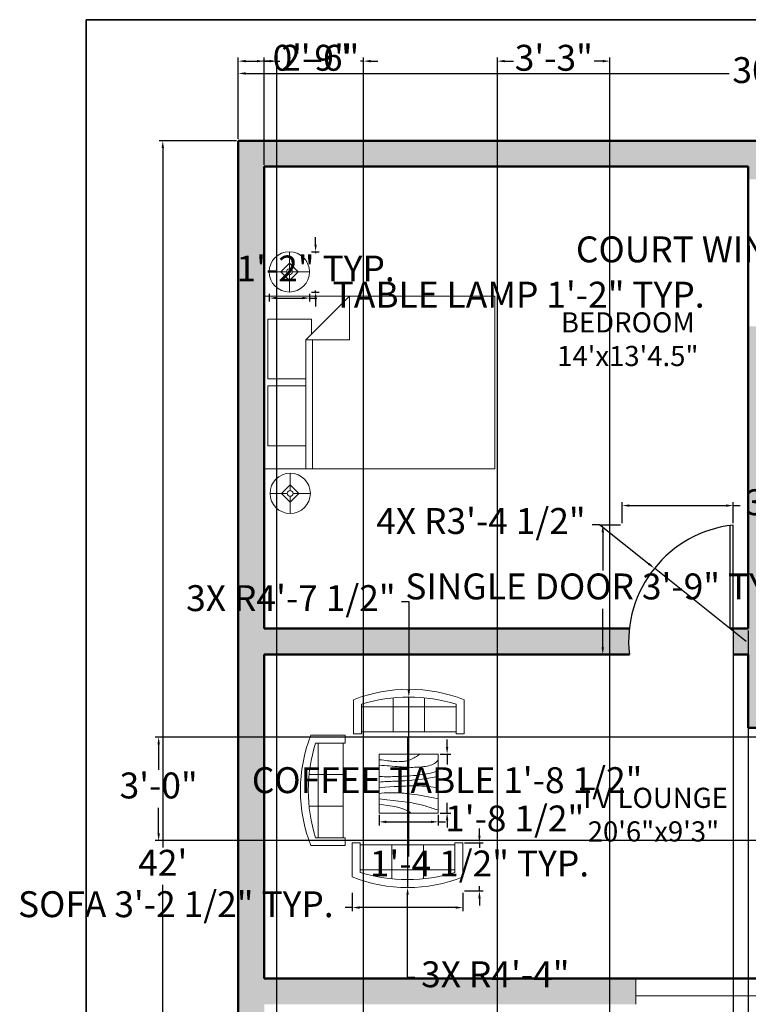
# Model space of a CAD drawing. Units: inches. Extents: x 3695 to 4182, y 4462 to 5050.
# Tile 2 of 3: x 3695 to 3948, y 4708 to 5050. Entities that reach past the tile are written whole.
import ezdxf

# ---------------------------------------------------------------- set-up
doc = ezdxf.new("R2010")
doc.units = ezdxf.units.IN
for name, color, linetype, lineweight in [('A-ANNO-DIMS', 2, 'Continuous', 18), ('A-ANNO-TTLB', 7, 'Continuous', 35), ('A-AREA-IDEN', 7, 'Continuous', 25), ('A-DOOR', 3, 'Continuous', 25), ('A-FURN', 8, 'Continuous', 18), ('A-GLAZ', 4, 'Continuous', 18), ('A-WALL', 7, 'Continuous', 50)]:
    doc.layers.add(name, color=color, linetype=linetype, lineweight=lineweight)
doc.layers.add('A-WALL-PATT', color=18, linetype='Continuous', lineweight=13, true_color=0x000000)
doc.styles.get("Standard").update_dxf_attribs({"font": 'arial.ttf'})
doc.dimstyles.new('ISO-25', dxfattribs={"dimtxt": 9, "dimasz": 2.5, "dimexe": 1.25, "dimexo": 0.625, "dimgap": 2, "dimtad": 0, "dimtih": 1, "dimtoh": 1, "dimdec": 1, "dimlunit": 4, "dimtxsty": 'Standard', "dimcen": 2.5, "dimadec": 0, "dimazin": 0, "dimtfac": 0.5, "dimtdec": 1, "dimtmove": 0, "dimatfit": 3, "dimfxl": 1, "dimarcsym": 0})

# ---------------------------------------------------------------- blocks, each defined once
blk = doc.blocks.new('Bed - Queen')
for p, q in [((0, -80.00003), (0, 0)), ((0, 0), (59.99999, 0)), ((59.99999, 0), (59.99999, -80.00003)), ((7.99999, -1.2), (28.79998, -1.2)), ((7.99999, -14.4), (7.99999, -1.2)), ((28.79998, -1.2), (28.79998, -14.4)), ((31.19999, -1.2), (51.99999, -1.2)), ((31.19999, -14.4), (31.19999, -1.2)), ((51.99999, -1.2), (51.99999, -16.4)), ((0, -14.4), (44.8, -14.4)), ((44.8, -16.8), (0, -16.8)), ((59.99999, -29.6), (44.8, -14.4)), ((44.8, -14.4), (44.8, -29.6)), ((51.99999, -16.4), (46.79936, -16.4)), ((44.8, -29.6), (59.99999, -29.6)), ((59.99999, -80.00003), (0, -80.00003))]:
    blk.add_line(p, q)
blk = doc.blocks.new('Sofa - Roundback 7 ft.')
for p, q in [((-12.00002, -32.4421), (-12.00003, -6.5971)), ((11.99997, -32.4421), (11.99998, -6.5971)), ((-36.000027, -34), (-36.000027, -11.4696)), ((-35.999844, -13.3819), (35.9998, -13.3819)), ((35.99998, -34), (35.99998, -11.4696)), ((-36.000027, -32.4421), (35.99998, -32.4421))]:
    blk.add_line(p, q)
for points in [[(-36.000027, -34), (-42.000027, -34), (-42.000027, -8)], [(41.99998, -8), (41.99998, -34), (35.99998, -34)]]:
    blk.add_lwpolyline(points)
for centre, radius, start, end in [((0, -114.25), 114.25, 68.43141, 111.5686), ((-0.00001, -127.1968), 121.1968, 72.72033, 107.2797)]:
    blk.add_arc(centre, radius, start, end)
blk = doc.blocks.new('Table - Square Woodgrain 42 x 42 in.')
blk.add_line((0, -42), (42, -42))
for points in [[(0, -4), (1.704, -4.2172), (3.2358, -4.4188), (4.615, -4.604), (5.8615, -4.7721), (6.9951, -4.9224), (8.0357, -5.0541), (9.0031, -5.1667), (9.9171, -5.2594), (10.7951, -5.3316), (11.6445, -5.3836), (12.4702, -5.4157), (13.277, -5.4283), (14.0698, -5.4217), (14.8535, -5.3964), (15.6331, -5.3526), (16.4133, -5.2908), (17.1986, -5.2103), (17.9913, -5.1062), (18.793, -4.9727), (19.6056, -4.8038), (20.4307, -4.5937), (21.2701, -4.3365), (22.1256, -4.0262), (22.9989, -3.6571), (23.888, -3.2272), (24.7756, -2.7516), (25.6408, -2.2491), (26.4624, -1.7387), (27.2195, -1.2395), (27.891, -0.7703), (28.456, -0.3501), (28.8934, 0.002)], [(0, -42), (0, 0), (42, 0), (42, -42)], [(0, -8), (1.8203, -8.1001), (3.6741, -8.2149), (5.5411, -8.3408), (7.4011, -8.4741), (9.2339, -8.6112), (11.0193, -8.7484), (12.7371, -8.8821), (14.3671, -9.0086), (15.8954, -9.1246), (17.3337, -9.2278), (18.6997, -9.3159), (20.0116, -9.387), (21.2871, -9.4389), (22.5442, -9.4696), (23.8008, -9.477), (25.0749, -9.459), (26.3791, -9.4137), (27.7049, -9.3403), (29.0383, -9.2382), (30.3655, -9.1068), (31.6728, -8.9455), (32.9461, -8.7535), (34.1717, -8.5304), (35.3358, -8.2756), (36.4268, -7.9863), (37.443, -7.6521), (38.3849, -7.2603), (39.253, -6.7986), (40.048, -6.2542), (40.7705, -5.6147), (41.421, -4.8674), (42, -4)], [(42, -12), (39.1784, -12.8621), (36.4519, -13.5654), (33.8246, -14.1294), (31.3004, -14.5731), (28.8832, -14.9161), (26.577, -15.1775), (24.3858, -15.3768), (22.3136, -15.5332), (20.3622, -15.6632), (18.5254, -15.7718), (16.7947, -15.8612), (15.1618, -15.9338), (13.6183, -15.9916), (12.1558, -16.0369), (10.7659, -16.0718), (9.4403, -16.0987), (8.1703, -16.1191), (6.9461, -16.1325), (5.7577, -16.1377), (4.595, -16.1335), (3.4479, -16.1188), (2.3064, -16.0924), (1.1604, -16.0532), (0, -16)], [(42, -16), (37.6529, -16.7365), (33.8802, -17.329), (30.6179, -17.7961), (27.8015, -18.1561), (25.3668, -18.4275), (23.2497, -18.6288), (21.3859, -18.7785), (19.7111, -18.8949), (18.1693, -18.9939), (16.7375, -19.0795), (15.401, -19.1534), (14.1449, -19.217), (12.9544, -19.2717), (11.8148, -19.3191), (10.7113, -19.3606), (9.6291, -19.3976), (8.5534, -19.4323), (7.47, -19.4689), (6.3643, -19.5122), (5.222, -19.5672), (4.0288, -19.6386), (2.7703, -19.7313), (1.4321, -19.8501), (0, -20)], [(0, -24), (3.9243, -23.6805), (7.4766, -23.4138), (10.6891, -23.1954), (13.5943, -23.0205), (16.2247, -22.8847), (18.6125, -22.7832), (20.7903, -22.7116), (22.7903, -22.6651), (24.6563, -22.642), (26.4764, -22.6507), (28.35, -22.7024), (30.3766, -22.8084), (32.6555, -22.98), (35.2861, -23.2283), (38.3678, -23.5645), (42, -24)], [(42, -32), (37.392, -31.017), (33.4585, -30.2231), (30.1291, -29.5949), (27.3334, -29.109), (25.0009, -28.742), (23.0612, -28.4707), (21.4439, -28.2716), (20.0786, -28.1215), (18.8998, -28.0002), (17.8609, -27.9014), (16.9206, -27.8219), (16.0371, -27.7588), (15.1691, -27.709), (14.2748, -27.6693), (13.3128, -27.6368), (12.2415, -27.6083), (11.0295, -27.5824), (9.6867, -27.5643), (8.233, -27.5608), (6.6884, -27.5787), (5.0728, -27.6248), (3.4062, -27.7058), (1.7086, -27.8286), (0, -28)], [(0, -32), (5.4026, -32.5358), (9.9494, -33.019), (13.7424, -33.4553), (16.8834, -33.8505), (19.4743, -34.2106), (21.6171, -34.5413), (23.4136, -34.8486), (24.9657, -35.1382), (26.3614, -35.4156), (27.6332, -35.6841), (28.7995, -35.9467), (29.8788, -36.2064), (30.8897, -36.4661), (31.8507, -36.7288), (32.7802, -36.9973), (33.6968, -37.2747), (34.6175, -37.5635), (35.5531, -37.8651), (36.5128, -38.1805), (37.506, -38.5108), (38.5421, -38.8568), (39.6302, -39.2197), (40.7797, -39.6004), (42, -40)], [(0, -36), (3.0098, -36.2857), (5.5354, -36.5643), (7.6368, -36.8359), (9.374, -37.1009), (10.807, -37.3597), (11.9957, -37.6126), (13.0002, -37.8599), (13.8804, -38.102), (14.6874, -38.3393), (15.4365, -38.5729), (16.1338, -38.8041), (16.7858, -39.0341), (17.3987, -39.264), (17.9787, -39.4952), (18.5322, -39.7288), (19.0655, -39.9662), (19.5832, -40.2081), (20.0842, -40.4544), (20.5657, -40.7046), (21.0249, -40.9581), (21.459, -41.2144), (21.8653, -41.4731), (22.2409, -41.7335), (22.5831, -41.9951)]]:
    blk.add_lwpolyline(points)
blk = doc.blocks.new('Lamp - Table')
for p, q in [((0, 7), (0, 1)), ((-1, 0), (-7, 0)), ((0, 3), (-3, 0)), ((-3, 0), (0, -3)), ((3, 0), (0, 3)), ((0, -3), (3, 0)), ((1, 0), (7, 0)), ((0, -1), (0, -7))]:
    blk.add_line(p, q)
for radius in [7, 1]:
    blk.add_circle((0, 0), radius)
blk = doc.blocks.new('*D11')
at = {"layer": 'A-ANNO-DIMS', "color": 0, "lineweight": -2, "transparency": 16777216}
for p, q in [((3770.96, 5008.15), (3770.96, 5032.15)), ((4130.96, 5008.15), (4130.96, 5032.15)), ((3773.46, 5030.9), (3941.33, 5030.9)), ((4128.46, 5030.9), (3960.6, 5030.9))]:
    blk.add_line(p, q, dxfattribs=at)
at = {"layer": 'A-ANNO-DIMS', "color": 0, "transparency": 16777216}
for points in [[(3773.46, 5031.31), (3773.46, 5030.48), (3770.96, 5030.9)], [(4128.46, 5031.31), (4128.46, 5030.48), (4130.96, 5030.9)]]:
    blk.add_solid(points, dxfattribs=at)
at = {"layer": 'Defpoints', "color": 0, "transparency": 16777216}
for p in [(4130.96, 5030.9), (3770.96, 5007.52), (4130.96, 5007.52)]:
    blk.add_point(p, dxfattribs=at)
at = {"layer": 'A-ANNO-DIMS', "color": 0, "transparency": 16777216, "insert": (3950.96, 5030.9), "char_height": 9, "attachment_point": 5}
blk.add_mtext("30'", dxfattribs=at)
blk = doc.blocks.new('*D12')
at = {"layer": 'A-ANNO-DIMS', "color": 0, "lineweight": -2, "transparency": 16777216}
for p, q in [((3770.34, 5007.52), (3743.5, 5007.52)), ((3744.75, 5005.02), (3744.75, 4762.04)), ((3744.75, 4506.02), (3744.75, 4749)), ((3770.34, 4503.52), (3743.5, 4503.52))]:
    blk.add_line(p, q, dxfattribs=at)
at = {"layer": 'A-ANNO-DIMS', "color": 0, "transparency": 16777216}
for points in [[(3744.34, 5005.02), (3745.17, 5005.02), (3744.75, 5007.52)], [(3744.34, 4506.02), (3745.17, 4506.02), (3744.75, 4503.52)]]:
    blk.add_solid(points, dxfattribs=at)
at = {"layer": 'Defpoints', "color": 0, "transparency": 16777216}
for p in [(3770.96, 5007.52), (3744.75, 4503.52), (3770.96, 4503.52)]:
    blk.add_point(p, dxfattribs=at)
at = {"layer": 'A-ANNO-DIMS', "color": 0, "transparency": 16777216, "insert": (3744.75, 4755.52), "char_height": 9, "attachment_point": 5}
blk.add_mtext("42'", dxfattribs=at)
blk = doc.blocks.new('DOOR-SINGLE-36IN')
for p, q in [((35.25, 9), (35.25, 45)), ((36.25, 9), (36.25, 45)), ((36.25, 9), (36.25, 0))]:
    blk.add_line(p, q)
blk.add_arc((40.75, 4.5), 40.75, 96.3402, 186.3402)
blk = doc.blocks.new('*D15')
at = {"layer": 'A-ANNO-DIMS', "color": 0, "lineweight": -2, "transparency": 16777216}
for p, q in [((3781.68, 4954.35), (3781.68, 4951.62)), ((3784.18, 4952.87), (3793.18, 4952.87)), ((3795.68, 4954.35), (3795.68, 4951.62)), ((3795.68, 4952.87), (3798.18, 4952.87))]:
    blk.add_line(p, q, dxfattribs=at)
at = {"layer": 'A-ANNO-DIMS', "color": 0, "transparency": 16777216}
for points in [[(3784.18, 4953.29), (3784.18, 4952.45), (3781.68, 4952.87)], [(3793.18, 4953.29), (3793.18, 4952.45), (3795.68, 4952.87)]]:
    blk.add_solid(points, dxfattribs=at)
at = {"layer": 'Defpoints', "color": 0, "transparency": 16777216}
for p in [(3781.68, 4954.97), (3795.68, 4954.97), (3795.68, 4952.87)]:
    blk.add_point(p, dxfattribs=at)
at = {"layer": 'A-ANNO-DIMS', "color": 0, "transparency": 16777216, "insert": (3868.25, 4952.87), "char_height": 9, "attachment_point": 5}
blk.add_mtext('TABLE LAMP 1\'-2" TYP.', dxfattribs=at)
blk = doc.blocks.new('*D16')
at = {"layer": 'A-ANNO-DIMS', "color": 0, "lineweight": -2, "transparency": 16777216}
for p, q in [((3797.78, 4971.47), (3797.78, 4973.97)), ((3796.31, 4968.97), (3799.03, 4968.97)), ((3797.78, 4968.97), (3797.78, 4968.49)), ((3796.31, 4954.97), (3799.03, 4954.97)), ((3797.78, 4954.97), (3797.78, 4955.45)), ((3797.78, 4952.47), (3797.78, 4949.97))]:
    blk.add_line(p, q, dxfattribs=at)
at = {"layer": 'A-ANNO-DIMS', "color": 0, "transparency": 16777216}
for points in [[(3797.37, 4971.47), (3798.2, 4971.47), (3797.78, 4968.97)], [(3797.37, 4952.47), (3798.2, 4952.47), (3797.78, 4954.97)]]:
    blk.add_solid(points, dxfattribs=at)
at = {"layer": 'Defpoints', "color": 0, "transparency": 16777216}
for p in [(3795.68, 4968.97), (3797.78, 4968.97), (3795.68, 4954.97)]:
    blk.add_point(p, dxfattribs=at)
at = {"layer": 'A-ANNO-DIMS', "color": 0, "transparency": 16777216, "insert": (3797.78, 4961.97), "char_height": 9, "attachment_point": 5}
blk.add_mtext('1\'-2" TYP.', dxfattribs=at)
blk = doc.blocks.new('*D17')
at = {"layer": 'A-ANNO-DIMS', "color": 0, "lineweight": -2, "transparency": 16777216}
for p, q in [((3903.58, 4874.02), (3896.2, 4874.02)), ((3897.45, 4871.52), (3897.45, 4858.18)), ((3897.45, 4831.52), (3897.45, 4844.86)), ((3903.58, 4829.02), (3896.2, 4829.02))]:
    blk.add_line(p, q, dxfattribs=at)
at = {"layer": 'A-ANNO-DIMS', "color": 0, "transparency": 16777216}
for points in [[(3897.04, 4871.52), (3897.87, 4871.52), (3897.45, 4874.02)], [(3897.04, 4831.52), (3897.87, 4831.52), (3897.45, 4829.02)]]:
    blk.add_solid(points, dxfattribs=at)
at = {"layer": 'Defpoints', "color": 0, "transparency": 16777216}
for p in [(3897.45, 4874.02), (3904.2, 4874.02), (3904.2, 4829.02)]:
    blk.add_point(p, dxfattribs=at)
at = {"layer": 'A-ANNO-DIMS', "color": 0, "transparency": 16777216, "insert": (3897.45, 4851.52), "char_height": 9, "attachment_point": 5}
blk.add_mtext('SINGLE DOOR 3\'-9" TYP.', dxfattribs=at)
blk = doc.blocks.new('*D18')
at = {"layer": 'A-ANNO-DIMS', "color": 0, "lineweight": -2, "transparency": 16777216}
for p, q in [((3904.2, 4874.65), (3904.2, 4882.02)), ((3942.69, 4874.65), (3942.69, 4882.02)), ((3906.7, 4880.77), (3940.19, 4880.77)), ((3942.69, 4880.77), (3945.19, 4880.77))]:
    blk.add_line(p, q, dxfattribs=at)
at = {"layer": 'A-ANNO-DIMS', "color": 0, "transparency": 16777216}
for points in [[(3906.7, 4881.19), (3906.7, 4880.36), (3904.2, 4880.77)], [(3940.19, 4881.19), (3940.19, 4880.36), (3942.69, 4880.77)]]:
    blk.add_solid(points, dxfattribs=at)
at = {"layer": 'Defpoints', "color": 0, "transparency": 16777216}
for p in [(3942.69, 4880.77), (3904.2, 4874.02), (3942.69, 4874.02)]:
    blk.add_point(p, dxfattribs=at)
at = {"layer": 'A-ANNO-DIMS', "color": 0, "transparency": 16777216, "insert": (3985.1, 4880.77), "char_height": 9, "attachment_point": 5}
blk.add_mtext('3\'-2 1/2" TYP.', dxfattribs=at)
blk = doc.blocks.new('*D19')
at = {"layer": 'A-ANNO-DIMS', "color": 0, "lineweight": -2, "transparency": 16777216}
for p, q in [((3810.53, 4746.26), (3810.53, 4739.88)), ((3848.89, 4746.26), (3848.89, 4739.88)), ((3810.53, 4741.13), (3808.03, 4741.13)), ((3846.39, 4741.13), (3813.03, 4741.13))]:
    blk.add_line(p, q, dxfattribs=at)
at = {"layer": 'A-ANNO-DIMS', "color": 0, "transparency": 16777216}
for points in [[(3813.03, 4741.55), (3813.03, 4740.72), (3810.53, 4741.13)], [(3846.39, 4741.55), (3846.39, 4740.72), (3848.89, 4741.13)]]:
    blk.add_solid(points, dxfattribs=at)
at = {"layer": 'Defpoints', "color": 0, "transparency": 16777216}
for p in [(3810.53, 4746.89), (3848.89, 4746.89), (3810.53, 4741.13)]:
    blk.add_point(p, dxfattribs=at)
at = {"layer": 'A-ANNO-DIMS', "color": 0, "transparency": 16777216, "insert": (3749.27, 4741.13), "char_height": 9, "attachment_point": 5}
blk.add_mtext('SOFA 3\'-2 1/2" TYP.', dxfattribs=at)
blk = doc.blocks.new('*D20')
at = {"layer": 'A-ANNO-DIMS', "color": 0, "lineweight": -2, "transparency": 16777216}
for p, q in [((3854.65, 4766.13), (3854.65, 4768.63)), ((3849.52, 4763.63), (3855.9, 4763.63)), ((3854.65, 4763.63), (3854.65, 4761.91)), ((3854.65, 4746.89), (3854.65, 4748.61)), ((3849.52, 4746.89), (3855.9, 4746.89)), ((3854.65, 4744.39), (3854.65, 4741.89))]:
    blk.add_line(p, q, dxfattribs=at)
at = {"layer": 'A-ANNO-DIMS', "color": 0, "transparency": 16777216}
for points in [[(3854.23, 4766.13), (3855.07, 4766.13), (3854.65, 4763.63)], [(3854.23, 4744.39), (3855.07, 4744.39), (3854.65, 4746.89)]]:
    blk.add_solid(points, dxfattribs=at)
at = {"layer": 'Defpoints', "color": 0, "transparency": 16777216}
for p in [(3848.89, 4763.63), (3848.89, 4746.89), (3854.65, 4746.89)]:
    blk.add_point(p, dxfattribs=at)
at = {"layer": 'A-ANNO-DIMS', "color": 0, "transparency": 16777216, "insert": (3854.65, 4755.26), "char_height": 9, "attachment_point": 5}
blk.add_mtext('1\'-4 1/2" TYP.', dxfattribs=at)
blk = doc.blocks.new('*D23')
at = {"layer": 'A-ANNO-DIMS', "color": 0, "lineweight": -2, "transparency": 16777216}
for p, q in [((3957.59, 4994.14), (3965.88, 4994.14)), ((3964.63, 4991.64), (3964.63, 4975.27)), ((3964.63, 4945.57), (3964.63, 4961.95)), ((3957.59, 4943.07), (3965.88, 4943.07))]:
    blk.add_line(p, q, dxfattribs=at)
at = {"layer": 'A-ANNO-DIMS', "color": 0, "transparency": 16777216}
for points in [[(3964.21, 4991.64), (3965.04, 4991.64), (3964.63, 4994.14)], [(3964.21, 4945.57), (3965.04, 4945.57), (3964.63, 4943.07)]]:
    blk.add_solid(points, dxfattribs=at)
at = {"layer": 'Defpoints', "color": 0, "transparency": 16777216}
for p in [(3956.96, 4994.14), (3964.63, 4994.14), (3956.96, 4943.07)]:
    blk.add_point(p, dxfattribs=at)
at = {"layer": 'A-ANNO-DIMS', "color": 0, "transparency": 16777216, "insert": (3964.63, 4968.61), "char_height": 9, "attachment_point": 5}
blk.add_mtext('COURT WINDOW 4\'-3" TYP.', dxfattribs=at)
blk = doc.blocks.new('*D29')
at = {"layer": 'A-ANNO-DIMS', "color": 0, "lineweight": -2, "transparency": 16777216}
for p, q in [((3843.43, 4796.96), (3843.43, 4799.46)), ((3840.98, 4794.46), (3844.68, 4794.46)), ((3843.43, 4794.46), (3843.43, 4790.88)), ((3843.43, 4773.98), (3843.43, 4777.56)), ((3840.98, 4773.98), (3844.68, 4773.98)), ((3843.43, 4771.48), (3843.43, 4768.98))]:
    blk.add_line(p, q, dxfattribs=at)
at = {"layer": 'A-ANNO-DIMS', "color": 0, "transparency": 16777216}
for points in [[(3843.01, 4796.96), (3843.85, 4796.96), (3843.43, 4794.46)], [(3843.01, 4771.48), (3843.85, 4771.48), (3843.43, 4773.98)]]:
    blk.add_solid(points, dxfattribs=at)
at = {"layer": 'Defpoints', "color": 0, "transparency": 16777216}
for p in [(3840.36, 4794.46), (3843.43, 4794.46), (3840.36, 4773.98)]:
    blk.add_point(p, dxfattribs=at)
at = {"layer": 'A-ANNO-DIMS', "color": 0, "transparency": 16777216, "insert": (3843.43, 4784.22), "char_height": 9, "attachment_point": 5}
blk.add_mtext('COFFEE TABLE 1\'-8 1/2"', dxfattribs=at)
blk = doc.blocks.new('*D30')
at = {"layer": 'A-ANNO-DIMS', "color": 0, "lineweight": -2, "transparency": 16777216}
for p, q in [((3819.87, 4773.35), (3819.87, 4769.66)), ((3840.36, 4773.35), (3840.36, 4769.66)), ((3822.37, 4770.91), (3837.86, 4770.91)), ((3840.36, 4770.91), (3842.86, 4770.91))]:
    blk.add_line(p, q, dxfattribs=at)
at = {"layer": 'A-ANNO-DIMS', "color": 0, "transparency": 16777216}
for points in [[(3822.37, 4771.32), (3822.37, 4770.49), (3819.87, 4770.91)], [(3837.86, 4771.32), (3837.86, 4770.49), (3840.36, 4770.91)]]:
    blk.add_solid(points, dxfattribs=at)
at = {"layer": 'Defpoints', "color": 0, "transparency": 16777216}
for p in [(3819.87, 4773.98), (3840.36, 4773.98), (3840.36, 4770.91)]:
    blk.add_point(p, dxfattribs=at)
at = {"layer": 'A-ANNO-DIMS', "color": 0, "transparency": 16777216, "insert": (3866.88, 4770.91), "char_height": 9, "attachment_point": 5}
blk.add_mtext('1\'-8 1/2"', dxfattribs=at)
blk = doc.blocks.new('*D33')
at = {"layer": 'A-ANNO-DIMS', "color": 0, "lineweight": -2, "transparency": 16777216}
for p, q in [((3770.96, 5008.15), (3770.96, 5036.42)), ((3773.46, 5035.17), (3777.46, 5035.17)), ((3779.96, 4999.15), (3779.96, 5036.42)), ((3779.96, 5035.17), (3782.46, 5035.17))]:
    blk.add_line(p, q, dxfattribs=at)
at = {"layer": 'A-ANNO-DIMS', "color": 0, "transparency": 16777216}
for points in [[(3773.46, 5035.59), (3773.46, 5034.76), (3770.96, 5035.17)], [(3777.46, 5035.59), (3777.46, 5034.76), (3779.96, 5035.17)]]:
    blk.add_solid(points, dxfattribs=at)
at = {"layer": 'Defpoints', "color": 0, "transparency": 16777216}
for p in [(3779.96, 5035.17), (3770.96, 5007.52), (3779.96, 4998.52)]:
    blk.add_point(p, dxfattribs=at)
at = {"layer": 'A-ANNO-DIMS', "color": 0, "transparency": 16777216, "insert": (3796.43, 5035.17), "char_height": 9, "attachment_point": 5}
blk.add_mtext('0\'-9"', dxfattribs=at)
blk = doc.blocks.new('*D37')
at = {"layer": 'A-ANNO-DIMS', "color": 0, "lineweight": -2, "transparency": 16777216}
for p, q in [((3860.96, 4580.15), (3860.96, 5036.42)), ((3863.46, 5035.17), (3866.51, 5035.17)), ((3897.46, 5035.17), (3894.42, 5035.17)), ((3899.96, 4580.15), (3899.96, 5036.42))]:
    blk.add_line(p, q, dxfattribs=at)
at = {"layer": 'A-ANNO-DIMS', "color": 0, "transparency": 16777216}
for points in [[(3863.46, 5035.59), (3863.46, 5034.76), (3860.96, 5035.17)], [(3897.46, 5035.59), (3897.46, 5034.76), (3899.96, 5035.17)]]:
    blk.add_solid(points, dxfattribs=at)
at = {"layer": 'Defpoints', "color": 0, "transparency": 16777216}
for p in [(3899.96, 5035.17), (3860.96, 4579.52), (3899.96, 4579.52)]:
    blk.add_point(p, dxfattribs=at)
at = {"layer": 'A-ANNO-DIMS', "color": 0, "transparency": 16777216, "insert": (3880.46, 5035.17), "char_height": 9, "attachment_point": 5}
blk.add_mtext('3\'-3"', dxfattribs=at)
blk = doc.blocks.new('*D40')
at = {"layer": 'A-ANNO-DIMS', "color": 0, "lineweight": -2, "transparency": 16777216}
for p, q in [((4025.34, 4800.38), (3742.06, 4800.38)), ((3743.31, 4797.88), (3743.31, 4788.98)), ((3743.31, 4766.88), (3743.31, 4775.78)), ((4025.34, 4764.38), (3742.06, 4764.38))]:
    blk.add_line(p, q, dxfattribs=at)
at = {"layer": 'A-ANNO-DIMS', "color": 0, "transparency": 16777216}
for points in [[(3742.9, 4797.88), (3743.73, 4797.88), (3743.31, 4800.38)], [(3742.9, 4766.88), (3743.73, 4766.88), (3743.31, 4764.38)]]:
    blk.add_solid(points, dxfattribs=at)
at = {"layer": 'Defpoints', "color": 0, "transparency": 16777216}
for p in [(3743.31, 4800.38), (4025.96, 4800.38), (4025.96, 4764.38)]:
    blk.add_point(p, dxfattribs=at)
at = {"layer": 'A-ANNO-DIMS', "color": 0, "transparency": 16777216, "insert": (3743.31, 4782.38), "char_height": 9, "attachment_point": 5}
blk.add_mtext('3\'-0"', dxfattribs=at)
blk = doc.blocks.new('*D42')
at = {"layer": 'A-ANNO-DIMS', "color": 0, "lineweight": -2, "transparency": 16777216}
for p, q in [((3942.69, 4837.4), (3942.69, 4474.62)), ((3947.96, 4837.4), (3947.96, 4474.62)), ((3940.19, 4475.87), (3937.69, 4475.87)), ((3942.69, 4475.87), (3947.96, 4475.87)), ((3950.46, 4475.87), (3952.96, 4475.87))]:
    blk.add_line(p, q, dxfattribs=at)
at = {"layer": 'A-ANNO-DIMS', "color": 0, "transparency": 16777216}
for points in [[(3940.19, 4476.29), (3940.19, 4475.46), (3942.69, 4475.87)], [(3950.46, 4476.29), (3950.46, 4475.46), (3947.96, 4475.87)]]:
    blk.add_solid(points, dxfattribs=at)
at = {"layer": 'Defpoints', "color": 0, "transparency": 16777216}
for p in [(3942.69, 4838.02), (3947.96, 4838.02), (3947.96, 4475.87)]:
    blk.add_point(p, dxfattribs=at)
at = {"layer": 'A-ANNO-DIMS', "color": 0, "transparency": 16777216, "insert": (3977.41, 4475.87), "char_height": 9, "attachment_point": 5}
blk.add_mtext('0\'-5 1/2"', dxfattribs=at)
blk = doc.blocks.new('*D45')
at = {"layer": 'A-ANNO-DIMS', "color": 0, "lineweight": -2, "transparency": 16777216}
for p, q in [((3781.88, 5035.17), (3779.38, 5035.17)), ((3784.38, 4580.15), (3784.38, 5036.42)), ((3784.38, 5035.17), (3785.34, 5035.17)), ((3814.38, 5035.17), (3813.42, 5035.17)), ((3814.38, 4580.15), (3814.38, 5036.42)), ((3816.88, 5035.17), (3819.38, 5035.17))]:
    blk.add_line(p, q, dxfattribs=at)
at = {"layer": 'A-ANNO-DIMS', "color": 0, "transparency": 16777216}
for points in [[(3781.88, 5035.59), (3781.88, 5034.76), (3784.38, 5035.17)], [(3816.88, 5035.59), (3816.88, 5034.76), (3814.38, 5035.17)]]:
    blk.add_solid(points, dxfattribs=at)
at = {"layer": 'Defpoints', "color": 0, "transparency": 16777216}
for p in [(3814.38, 5035.17), (3784.38, 4579.52), (3814.38, 4579.52)]:
    blk.add_point(p, dxfattribs=at)
at = {"layer": 'A-ANNO-DIMS', "color": 0, "transparency": 16777216, "insert": (3799.38, 5035.17), "char_height": 9, "attachment_point": 5}
blk.add_mtext('2\'-6"', dxfattribs=at)
blk = doc.blocks.new('*D52')
at = {"layer": 'A-ANNO-DIMS', "color": 0, "lineweight": -2, "transparency": 16777216}
for p, q in [((3827.63, 4847.46), (3830.13, 4847.46)), ((3830.13, 4847.46), (3830.13, 4816.74)), ((3830.13, 4758.88), (3830.13, 4814.24))]:
    blk.add_line(p, q, dxfattribs=at)
at = {"layer": 'A-ANNO-DIMS', "color": 0, "transparency": 16777216}
blk.add_solid([(3830.55, 4816.74), (3829.71, 4816.74), (3830.13, 4814.24)], dxfattribs=at)
at = {"layer": 'Defpoints', "color": 0, "transparency": 16777216}
for p in [(3830.13, 4814.24), (3830.13, 4758.88)]:
    blk.add_point(p, dxfattribs=at)
at = {"layer": 'A-ANNO-DIMS', "color": 0, "transparency": 16777216, "insert": (3789.21, 4847.46), "char_height": 9, "attachment_point": 5}
blk.add_mtext('3X R4\'-7 1/2"', dxfattribs=at)
blk = doc.blocks.new('*D53')
at = {"layer": 'A-ANNO-DIMS', "color": 0, "lineweight": -2, "transparency": 16777216}
for p, q in [((3829.71, 4800.29), (3829.71, 4748.1)), ((3829.71, 4716.79), (3829.71, 4745.6)), ((3832.21, 4716.79), (3829.71, 4716.79))]:
    blk.add_line(p, q, dxfattribs=at)
at = {"layer": 'A-ANNO-DIMS', "color": 0, "transparency": 16777216}
blk.add_solid([(3830.13, 4745.6), (3829.29, 4745.6), (3829.71, 4748.1)], dxfattribs=at)
at = {"layer": 'Defpoints', "color": 0, "transparency": 16777216}
for p in [(3829.71, 4800.29), (3829.71, 4748.1)]:
    blk.add_point(p, dxfattribs=at)
at = {"layer": 'A-ANNO-DIMS', "color": 0, "transparency": 16777216, "insert": (3860.15, 4716.79), "char_height": 9, "attachment_point": 5}
blk.add_mtext('3X R4\'-4"', dxfattribs=at)
blk = doc.blocks.new('*D54')
at = {"layer": 'A-ANNO-DIMS', "color": 0, "lineweight": -2, "transparency": 16777216}
for p, q in [((3893.78, 4874.25), (3896.28, 4874.25)), ((3896.28, 4874.25), (3913.42, 4860.54)), ((3947.19, 4833.52), (3915.37, 4858.98))]:
    blk.add_line(p, q, dxfattribs=at)
at = {"layer": 'A-ANNO-DIMS', "color": 0, "transparency": 16777216}
blk.add_solid([(3913.68, 4860.87), (3913.16, 4860.22), (3915.37, 4858.98)], dxfattribs=at)
at = {"layer": 'Defpoints', "color": 0, "transparency": 16777216}
for p in [(3915.37, 4858.98), (3947.19, 4833.52)]:
    blk.add_point(p, dxfattribs=at)
at = {"layer": 'A-ANNO-DIMS', "color": 0, "transparency": 16777216, "insert": (3855.17, 4874.25), "char_height": 9, "attachment_point": 5}
blk.add_mtext('4X R3\'-4 1/2"', dxfattribs=at)

msp = doc.modelspace()

# ---------------------------------------------------------------- hatches: boundary and pattern name
at = {"layer": 'A-WALL-PATT'}
h = msp.add_hatch(color=256, dxfattribs=at)
h.dxf.hatch_style = 1
h.paths.add_polyline_path([(3906.69, 4838.02), (3779.96, 4838.02), (3779.96, 4998.52), (3947.96, 4998.52), (3947.96, 4994.14), (3956.96, 4994.14), (3956.96, 4998.52), (4016.96, 4998.52), (4016.96, 4994.14), (4025.96, 4994.14), (4025.96, 4998.52), (4121.96, 4998.52), (4121.96, 4938.52), (4118.4, 4938.52), (4118.4, 4932.52), (4121.96, 4932.52), (4121.96, 4812.52), (4025.96, 4812.52), (3998.16, 4812.52, -0.055385), (3998.16, 4803.52), (4025.96, 4803.52), (4025.96, 4800.38), (4034.96, 4800.38), (4034.96, 4803.52), (4121.96, 4803.52), (4121.96, 4716.52), (4103.96, 4716.52), (4103.96, 4707.52), (4121.96, 4707.52), (4121.96, 4512.52), (4111.49, 4512.52), (4111.49, 4503.52), (4130.96, 4503.52), (4130.96, 5007.52), (3770.96, 5007.52), (3770.96, 4503.52), (4004.7, 4503.52), (4004.7, 4512.52), (3860.96, 4512.52), (3860.96, 4529.52), (3851.96, 4529.52), (3851.96, 4512.52), (3779.96, 4512.52), (3779.96, 4570.52), (3784.38, 4570.52), (3784.38, 4579.52), (3779.96, 4579.52), (3779.96, 4707.52), (3908.96, 4707.52), (3908.96, 4716.52), (3779.96, 4716.52), (3779.96, 4829.02), (3906.69, 4829.02, -0.055385)])
h.paths.add_polyline_path([(4034.96, 4764.38, -0.055385), (4025.96, 4764.38), (4025.96, 4716.52), (4025.96, 4707.52), (4043.96, 4707.52), (4043.96, 4716.52), (4034.96, 4716.52)], flags=17)
h = msp.add_hatch(color=256, dxfattribs=at)
h.dxf.hatch_style = 1
h.paths.add_polyline_path([(3956.96, 4932.52), (3960.75, 4932.52), (3960.75, 4938.52), (3956.96, 4938.52), (3956.96, 4943.07), (3947.96, 4943.07), (3947.96, 4838.02), (3942.69, 4838.02), (3942.69, 4829.02), (3947.96, 4829.02), (3947.96, 4803.52), (3956.96, 4803.52), (3962.16, 4803.52), (3962.16, 4812.52), (3956.96, 4812.52), (3956.96, 4829.02)])
h.paths.add_polyline_path([(4088.4, 4938.52), (4025.96, 4938.52), (4025.96, 4943.07), (4016.96, 4943.07), (4016.96, 4938.52), (4012.55, 4938.52), (4012.55, 4932.52), (4057.18, 4932.52), (4088.4, 4932.52, -0.045361)])

# ---------------------------------------------------------------- linework, layer by layer
at = {"layer": 'A-ANNO-TTLB'}
msp.add_lwpolyline([(3718.2, 5049.57), (4146.02, 5049.57), (4146.02, 4481.47), (3718.2, 4481.47)], close=True, dxfattribs=at)
at = {"layer": 'A-GLAZ'}
for p, q in [((3908.96, 4707.52), (3908.96, 4716.52)), ((4025.96, 4710.52), (3908.96, 4710.52))]:
    msp.add_line(p, q, dxfattribs=at)
at = {"layer": 'A-WALL'}
for p, q in [((3770.96, 5007.52), (4130.96, 5007.52)), ((3770.96, 4503.52), (3770.96, 5007.52)), ((3779.96, 4998.52), (3947.96, 4998.52)), ((3779.96, 4838.02), (3779.96, 4998.52)), ((3947.96, 4838.02), (3947.96, 4998.52)), ((3779.96, 4838.02), (3906.69, 4838.02)), ((3941.69, 4838.02), (3947.96, 4838.02)), ((3779.96, 4829.02), (3906.69, 4829.02)), ((3779.96, 4716.52), (3779.96, 4829.02)), ((3942.69, 4829.02), (3947.96, 4829.02)), ((3947.96, 4829.02), (3947.96, 4803.52)), ((3956.96, 4803.52), (3947.96, 4803.52)), ((4025.96, 4716.52), (3779.96, 4716.52))]:
    msp.add_line(p, q, dxfattribs=at)

# ---------------------------------------------------------------- block references
at = {"layer": 'A-DOOR'}
msp.add_blockref('DOOR-SINGLE-36IN', (3906.44, 4829.02), dxfattribs=at)
at = {"layer": 'A-FURN'}
for p in [(3788.68, 4961.97), (3788.97, 4885.01)]:
    msp.add_blockref('Lamp - Table', p, dxfattribs=at)
at = {"layer": 'A-FURN', "rotation": 89.99999999999999}
msp.add_blockref('Bed - Queen', (3779.96, 4893.56), dxfattribs=at)
at = {"layer": 'A-FURN'}
for name, p, xscale, yscale, zscale in [('Sofa - Roundback 7 ft.', (3830.13, 4816.98), 0.4567606886891789, 0.4567606886891789, 0.4567606886891789), ('Table - Square Woodgrain 42 x 42 in.', (3819.87, 4794.46), 0.4877277078007204, 0.4877277078007204, 0.4877277078007204)]:
    msp.add_blockref(name, p, dxfattribs=dict(at, xscale=xscale, yscale=yscale, zscale=zscale))
at = {"layer": 'A-FURN', "xscale": 0.4567606886891789, "yscale": 0.4567606886891789, "zscale": 0.4567606886891789}
for p, rotation in [((3792.51, 4781.85), 90), ((3829.71, 4748.1), 180)]:
    msp.add_blockref('Sofa - Roundback 7 ft.', p, dxfattribs=dict(at, rotation=rotation))

# ---------------------------------------------------------------- texts
at = {"layer": 'A-AREA-IDEN', "char_height": 7, "attachment_point": 1}
for s, width, insert in [('\\pxqc;{\\fArial|b1|i0|c0|p34;BEDROOM\\P14\'x13\'4.5"}', 69.4443, (3871.43, 4947.92)), ('\\pxqc;{\\fArial|b1|i0|c0|p34;TV LOUNGE\\P20\'6"x9\'3"}', 83.0367, (3873.52, 4782.75))]:
    msp.add_mtext_dynamic_manual_height_columns(s, width=width, gutter_width=12.5, heights=[0], dxfattribs=dict(at, insert=insert))

# ---------------------------------------------------------------- dimensions: what is measured, and where the dimension line sits
at = {"layer": 'A-ANNO-DIMS'}
for base, p1, p2, override, picture, middle in [((3779.96, 5035.17), (3770.96, 5007.52), (3779.96, 4998.52), {"dimdec": 1, "dimlfac": 1, "dimrnd": 0, "dimzin": 1, "dimdsep": 46, "dimlunit": 4, "dimfrac": 2}, '*D33', (3796.43, 5035.17)), ((3814.38, 5035.17), (3784.38, 4579.52), (3814.38, 4579.52), {"dimdec": 1, "dimlfac": 1, "dimrnd": 0, "dimzin": 1, "dimdsep": 46, "dimlunit": 4, "dimfrac": 2}, '*D45', (3799.38, 5035.17)), ((3899.96, 5035.17), (3860.96, 4579.52), (3899.96, 4579.52), {"dimdec": 1, "dimlfac": 1, "dimrnd": 0, "dimzin": 1, "dimdsep": 46, "dimlunit": 4, "dimfrac": 2}, '*D37', (3880.46, 5035.17)), ((4130.96, 5030.9), (3770.96, 5007.52), (4130.96, 5007.52), {"dimclrd": 0, "dimclre": 0, "dimclrt": 0}, '*D11', (3950.96, 5030.9)), ((3947.96, 4475.87), (3942.69, 4838.02), (3947.96, 4838.02), {"dimdec": 1, "dimlfac": 1, "dimrnd": 0, "dimzin": 1, "dimdsep": 46, "dimlunit": 4, "dimfrac": 2}, '*D42', (3977.41, 4475.87)), ((3840.36, 4770.91), (3819.87, 4773.98), (3840.36, 4773.98), {"dimdec": 1, "dimlfac": 1, "dimrnd": 0, "dimzin": 1, "dimdsep": 46, "dimlunit": 4, "dimfrac": 2}, '*D30', (3866.88, 4770.91))]:
    dim = msp.add_linear_dim(base=base, p1=p1, p2=p2, dimstyle='ISO-25', override=override, dxfattribs=at)
    dim.commit()
    dim.dimension.update_dxf_attribs({"geometry": picture, "text_midpoint": middle})
for base, p1, p2, override, picture, middle in [((3744.75, 4503.52), (3770.96, 5007.52), (3770.96, 4503.52), {"dimclrd": 0, "dimclre": 0, "dimclrt": 0}, '*D12', (3744.75, 4755.52)), ((3743.31, 4800.38), (4025.96, 4764.38), (4025.96, 4800.38), {"dimdec": 1, "dimlfac": 1, "dimrnd": 0, "dimzin": 1, "dimdsep": 46, "dimlunit": 4, "dimfrac": 2}, '*D40', (3743.31, 4782.38))]:
    dim = msp.add_linear_dim(base=base, p1=p1, p2=p2, angle=90, dimstyle='ISO-25', override=override, dxfattribs=at)
    dim.commit()
    dim.dimension.update_dxf_attribs({"geometry": picture, "text_midpoint": middle})
for base, p1, p2, angle, text, picture, middle in [((3964.63, 4994.14), (3956.96, 4943.07), (3956.96, 4994.14), 90, 'COURT WINDOW <> TYP.', '*D23', (3964.63, 4968.61)), ((3797.78, 4968.97), (3795.68, 4954.97), (3795.68, 4968.97), 90, '<> TYP.', '*D16', (3797.78, 4961.97)), ((3897.45, 4874.02), (3904.2, 4829.02), (3904.2, 4874.02), 90, 'SINGLE DOOR <> TYP.', '*D17', (3897.45, 4851.52)), ((3843.43, 4794.46), (3840.36, 4773.98), (3840.36, 4794.46), 90, 'COFFEE TABLE <>', '*D29', (3843.43, 4784.22)), ((3854.65, 4746.89), (3848.89, 4763.63), (3848.89, 4746.89), 270, '<> TYP.', '*D20', (3854.65, 4755.26)), ((3810.53, 4741.13), (3848.89, 4746.89), (3810.53, 4746.89), 180, 'SOFA <> TYP.', '*D19', (3749.27, 4741.13))]:
    dim = msp.add_linear_dim(base=base, p1=p1, p2=p2, angle=angle, text=text, dimstyle='ISO-25', override={"dimdec": 1, "dimlfac": 1, "dimrnd": 0, "dimzin": 1, "dimdsep": 46, "dimlunit": 4, "dimfrac": 2}, dxfattribs=at)
    dim.commit()
    dim.dimension.update_dxf_attribs({"geometry": picture, "text_midpoint": middle})
for base, p1, p2, text, picture, middle in [((3795.68, 4952.87), (3781.68, 4954.97), (3795.68, 4954.97), 'TABLE LAMP <> TYP.', '*D15', (3868.25, 4952.87)), ((3942.69, 4880.77), (3904.2, 4874.02), (3942.69, 4874.02), '<> TYP.', '*D18', (3985.1, 4880.77))]:
    dim = msp.add_linear_dim(base=base, p1=p1, p2=p2, text=text, dimstyle='ISO-25', override={"dimdec": 1, "dimlfac": 1, "dimrnd": 0, "dimzin": 1, "dimdsep": 46, "dimlunit": 4, "dimfrac": 2}, dxfattribs=at)
    dim.commit()
    dim.dimension.update_dxf_attribs({"geometry": picture, "text_midpoint": middle})
for center, mpoint, text, picture, middle in [((3947.1899, 4833.5232), (3915.37, 4858.979), '4X <>', '*D54', (3855.1734, 4874.2525)), ((3830.13, 4758.88), (3830.13, 4814.24), '3X <>', '*D52', (3789.21, 4847.46)), ((3829.71, 4800.29), (3829.71, 4748.1), '3X <>', '*D53', (3860.15, 4716.79))]:
    dim = msp.add_radius_dim(center=center, mpoint=mpoint, text=text, dimstyle='ISO-25', override={"dimdec": 1, "dimlfac": 1, "dimrnd": 0, "dimzin": 1, "dimdsep": 46, "dimlunit": 4, "dimfrac": 2}, dxfattribs=at)
    dim.commit()
    dim.dimension.update_dxf_attribs({"geometry": picture, "text_midpoint": middle, "dimtype": 164})

doc.saveas('drawing.dxf')
